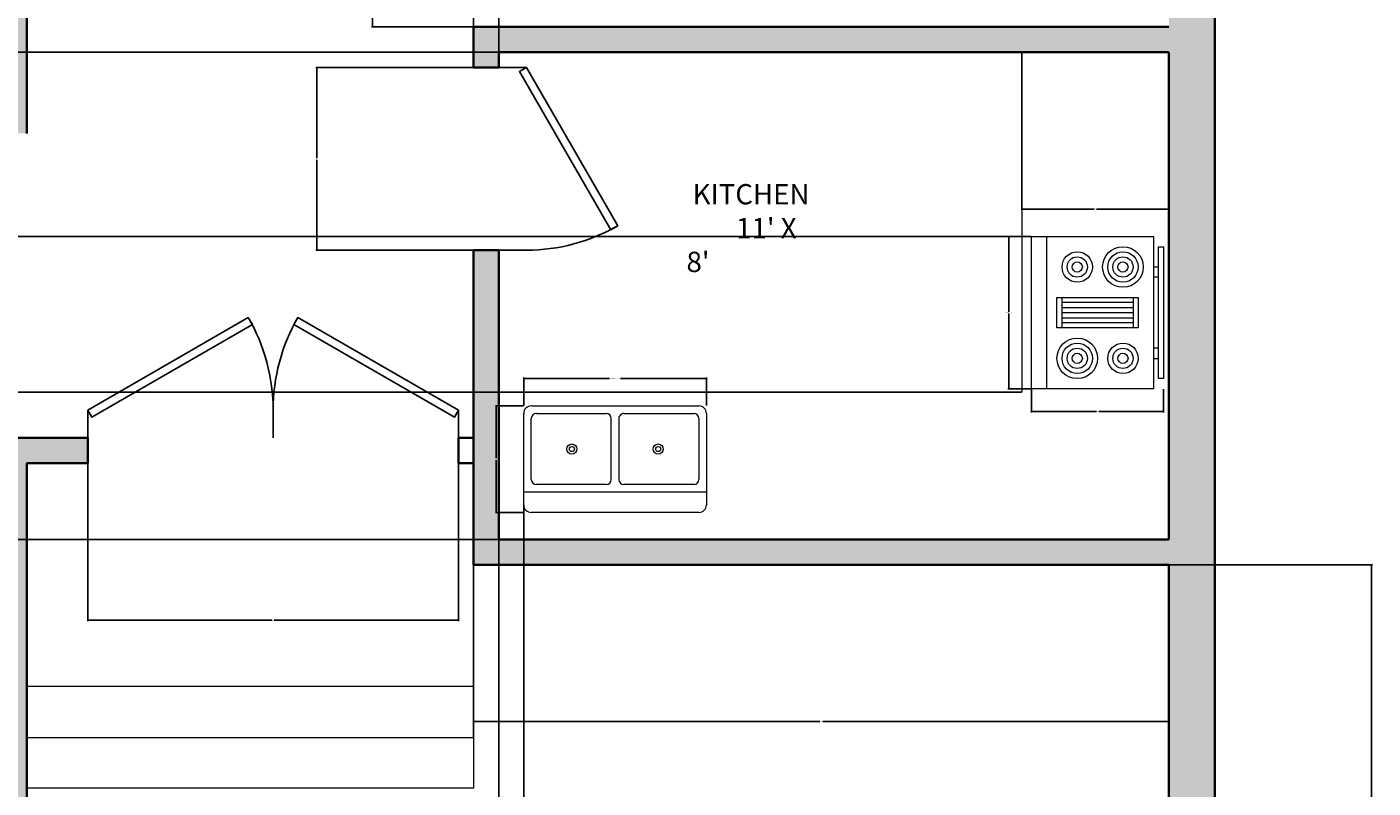
# Model space of a CAD drawing. Units: inches. Extents: x -30 to 437, y -29 to 647.
# Tile 6 of 15: x 172 to 437, y 105 to 255. Entities that reach past the tile are written whole.
import ezdxf

# ---------------------------------------------------------------- set-up
doc = ezdxf.new("R2010")
doc.units = ezdxf.units.IN
doc.header["$MEASUREMENT"] = 0
for name, color, linetype, lineweight in [('A-ANNO-DIMS', 2, 'Continuous', 18), ('A-AREA-IDEN', 7, 'Continuous', 18), ('A-FLOR-STRS', 7, 'Continuous', 18), ('A-WALL', 7, 'Continuous', 35), ('doors', 40, 'Continuous', 25), ('kitchen', 181, 'Continuous', 18)]:
    doc.layers.add(name, color=color, linetype=linetype, lineweight=lineweight)
doc.layers.add('A-WALL-PATT', color=251, linetype='Continuous', lineweight=13, true_color=0x636466)
doc.styles.get("Standard").update_dxf_attribs({"font": 'arial.ttf'})
doc.dimstyles.get("Standard").update_dxf_attribs({"dimtxt": 0.18, "dimasz": 0.18, "dimexe": 0.18, "dimexo": 0.0625, "dimgap": 0.09, "dimtad": 0, "dimtih": 1, "dimtoh": 1, "dimdec": 4, "dimzin": 0, "dimdsep": 46, "dimtxsty": 'Standard', "dimcen": 0.09, "dimadec": 0, "dimazin": 0, "dimtfac": 1, "dimtdec": 4, "dimtofl": 0, "dimtmove": 0, "dimatfit": 3, "dimfxl": 1, "dimtolj": 1, "dimtzin": 0, "dimarcsym": 0})

# ---------------------------------------------------------------- blocks, each defined once
blk = doc.blocks.new('*U6')
for p, q in [((0, 0), (0, -6)), ((40, 0), (40, -6))]:
    blk.add_line(p, q)
blk.add_lwpolyline([(0, 0), (34.64, 20), (35.52, 18.48), (0.87, -1.52)], close=True)
blk.add_arc((0, 0), 40, 0, 30)
blk = doc.blocks.new('Range-Oven - 30 in top')
for p, q in [((0, -3), (30, -3)), ((12, -6), (18, -6)), ((13, -20), (13, -6)), ((14, -6), (14, -20)), ((15, -20), (15, -6)), ((16, -6), (16, -20)), ((17, -20), (17, -6)), ((18, -20), (12, -20)), ((6, -24), (6, -25)), ((8, -25), (8, -24)), ((22, -25), (22, -24)), ((24, -24), (24, -25))]:
    blk.add_line(p, q)
for points in [[(0, -24), (0, 0), (30, 0), (30, -24)], [(12, -21), (12, -5), (18, -5), (18, -21)], [(2, -26), (2, -25), (28, -25), (28, -26)]]:
    blk.add_lwpolyline(points, close=True)
for centre, radius in [((6, -9), 4), ((6, -9), 3), ((6, -9), 2), ((24, -9), 3), ((24, -9), 2), ((6, -9), 1), ((24, -9), 1), ((6, -18), 3), ((24, -18), 4), ((24, -18), 3), ((6, -18), 2), ((6, -18), 1), ((24, -18), 2), ((24, -18), 1)]:
    blk.add_circle(centre, radius)
blk = doc.blocks.new('Sink-double - 36 in top')
for p, q in [((-18, -4), (18, -4)), ((-0.75, -18.5), (-0.75, -6.5)), ((0.75, -6.5), (0.75, -18.5))]:
    blk.add_line(p, q)
for points in [[(-16.5, 0), (16.5, 0)], [(-18, -19.5), (-18, -1.5)], [(18, -1.5), (18, -19.5)], [(-16.5, -18.5), (-16.5, -6.5)], [(-15.5, -5.5), (-1.75, -5.5)], [(1.75, -5.5), (15.5, -5.5)], [(16.5, -6.5), (16.5, -18.5)], [(16.5, -21), (-16.5, -21)], [(-1.75, -19.5), (-15.5, -19.5)], [(15.5, -19.5), (1.75, -19.5)]]:
    blk.add_lwpolyline(points)
for centre, radius in [((-8.5, -12.5), 1), ((-8.5, -12.5), 0.5), ((8.5, -12.5), 1), ((8.5, -12.5), 0.5)]:
    blk.add_circle(centre, radius)
for centre, radius, start, end in [((-16.5, -1.5), 1.5, 90, 180), ((16.5, -1.5), 1.5, 0, 90), ((-15.5, -6.5), 1, 90, 180), ((-1.75, -6.5), 1, 0, 90), ((1.75, -6.5), 1, 90, 180), ((15.5, -6.5), 1, 0, 90), ((-15.5, -18.5), 1, 180, 270), ((-1.75, -18.5), 1, 270, 0), ((1.75, -18.5), 1, 180, 270), ((15.5, -18.5), 1, 270, 0), ((-16.5, -19.5), 1.5, 180, 270), ((16.5, -19.5), 1.5, 270, 0)]:
    blk.add_arc(centre, radius, start, end)
blk = doc.blocks.new('*D21')
at = {"layer": 'A-ANNO-DIMS', "color": 0, "lineweight": -2, "transparency": 16777216}
for p, q in [((369.54, 213.24), (364.93, 213.24)), ((365.11, 213.06), (365.11, 198.42)), ((365.11, 183.42), (365.11, 198.05)), ((369.54, 183.24), (364.93, 183.24))]:
    blk.add_line(p, q, dxfattribs=at)
at = {"layer": 'A-ANNO-DIMS', "color": 0, "transparency": 16777216}
for points in [[(365.08, 213.06), (365.14, 213.06), (365.11, 213.24)], [(365.08, 183.42), (365.14, 183.42), (365.11, 183.24)]]:
    blk.add_solid(points, dxfattribs=at)
at = {"layer": 'Defpoints', "color": 0, "transparency": 16777216}
for p in [(365.11, 213.24), (369.61, 213.24), (369.61, 183.24)]:
    blk.add_point(p, dxfattribs=at)
at = {"layer": 'A-ANNO-DIMS', "color": 0, "transparency": 16777216, "insert": (365.11, 198.24), "char_height": 0.18, "attachment_point": 5}
blk.add_mtext('\\A1;RANGE 30', dxfattribs=at)
blk = doc.blocks.new('*D22')
at = {"layer": 'A-ANNO-DIMS', "color": 0, "lineweight": -2, "transparency": 16777216}
for p, q in [((369.61, 183.17), (369.61, 178.56)), ((395.61, 183.17), (395.61, 178.56)), ((369.79, 178.74), (382.39, 178.74)), ((395.43, 178.74), (382.83, 178.74))]:
    blk.add_line(p, q, dxfattribs=at)
at = {"layer": 'A-ANNO-DIMS', "color": 0, "transparency": 16777216}
for points in [[(369.79, 178.77), (369.79, 178.71), (369.61, 178.74)], [(395.43, 178.77), (395.43, 178.71), (395.61, 178.74)]]:
    blk.add_solid(points, dxfattribs=at)
at = {"layer": 'Defpoints', "color": 0, "transparency": 16777216}
for p in [(369.61, 183.24), (395.61, 183.24), (369.61, 178.74)]:
    blk.add_point(p, dxfattribs=at)
at = {"layer": 'A-ANNO-DIMS', "color": 0, "transparency": 16777216, "insert": (382.61, 178.74), "char_height": 0.18, "attachment_point": 5}
blk.add_mtext('\\A1;26', dxfattribs=at)
blk = doc.blocks.new('*D23')
at = {"layer": 'A-ANNO-DIMS', "color": 0, "lineweight": -2, "transparency": 16777216}
for p, q in [((269.54, 179.93), (269.54, 185.45)), ((269.72, 185.27), (286.45, 185.27)), ((305.36, 185.27), (288.64, 185.27)), ((305.54, 179.93), (305.54, 185.45))]:
    blk.add_line(p, q, dxfattribs=at)
at = {"layer": 'A-ANNO-DIMS', "color": 0, "transparency": 16777216}
for points in [[(269.72, 185.3), (269.72, 185.24), (269.54, 185.27)], [(305.36, 185.3), (305.36, 185.24), (305.54, 185.27)]]:
    blk.add_solid(points, dxfattribs=at)
at = {"layer": 'Defpoints', "color": 0, "transparency": 16777216}
for p in [(269.54, 185.27), (269.54, 179.87), (305.54, 179.87)]:
    blk.add_point(p, dxfattribs=at)
at = {"layer": 'A-ANNO-DIMS', "color": 0, "transparency": 16777216, "insert": (287.54, 185.27), "char_height": 0.18, "attachment_point": 5}
blk.add_mtext('\\A1;DOUBLE SINK 36', dxfattribs=at)
blk = doc.blocks.new('*D24')
at = {"layer": 'A-ANNO-DIMS', "color": 0, "lineweight": -2, "transparency": 16777216}
for p, q in [((269.48, 179.87), (263.96, 179.87)), ((264.14, 179.69), (264.14, 169.55)), ((264.14, 159.05), (264.14, 169.19)), ((269.48, 158.87), (263.96, 158.87))]:
    blk.add_line(p, q, dxfattribs=at)
at = {"layer": 'A-ANNO-DIMS', "color": 0, "transparency": 16777216}
for points in [[(264.11, 179.69), (264.17, 179.69), (264.14, 179.87)], [(264.11, 159.05), (264.17, 159.05), (264.14, 158.87)]]:
    blk.add_solid(points, dxfattribs=at)
at = {"layer": 'Defpoints', "color": 0, "transparency": 16777216}
for p in [(269.54, 179.87), (264.14, 158.87), (269.54, 158.87)]:
    blk.add_point(p, dxfattribs=at)
at = {"layer": 'A-ANNO-DIMS', "color": 0, "transparency": 16777216, "insert": (264.14, 169.37), "char_height": 0.18, "attachment_point": 5}
blk.add_mtext('\\A1;21', dxfattribs=at)
blk = doc.blocks.new('*D37')
at = {"layer": 'A-ANNO-DIMS', "color": 0, "lineweight": -2, "transparency": 16777216}
for p, q in [((259.67, 148.48), (259.67, 117.47)), ((396.67, 148.48), (396.67, 117.47)), ((259.85, 117.65), (327.89, 117.65)), ((396.49, 117.65), (328.45, 117.65))]:
    blk.add_line(p, q, dxfattribs=at)
at = {"layer": 'A-ANNO-DIMS', "color": 0, "transparency": 16777216}
for points in [[(259.85, 117.68), (259.85, 117.62), (259.67, 117.65)], [(396.49, 117.68), (396.49, 117.62), (396.67, 117.65)]]:
    blk.add_solid(points, dxfattribs=at)
at = {"layer": 'Defpoints', "color": 0, "transparency": 16777216}
for p in [(259.67, 148.55), (396.67, 148.55), (259.67, 117.65)]:
    blk.add_point(p, dxfattribs=at)
at = {"layer": 'A-ANNO-DIMS', "color": 0, "transparency": 16777216, "insert": (328.17, 117.65), "char_height": 0.18, "attachment_point": 5}
blk.add_mtext('\\A1;137', dxfattribs=at)
blk = doc.blocks.new('*D39')
at = {"layer": 'A-ANNO-DIMS', "color": 0, "lineweight": -2, "transparency": 16777216}
for p, q in [((396.74, 148.55), (436.75, 148.55)), ((436.57, 148.37), (436.57, 75.48)), ((436.57, 2.23), (436.57, 75.12)), ((396.74, 2.05), (436.75, 2.05))]:
    blk.add_line(p, q, dxfattribs=at)
at = {"layer": 'A-ANNO-DIMS', "color": 0, "transparency": 16777216}
for points in [[(436.54, 148.37), (436.6, 148.37), (436.57, 148.55)], [(436.54, 2.23), (436.6, 2.23), (436.57, 2.05)]]:
    blk.add_solid(points, dxfattribs=at)
at = {"layer": 'Defpoints', "color": 0, "transparency": 16777216}
for p in [(396.67, 148.55), (436.57, 148.55), (396.67, 2.05)]:
    blk.add_point(p, dxfattribs=at)
at = {"layer": 'A-ANNO-DIMS', "color": 0, "transparency": 16777216, "insert": (436.57, 75.3), "char_height": 0.18, "attachment_point": 5}
blk.add_mtext('\\A1;146.5', dxfattribs=at)
blk = doc.blocks.new('*D41')
at = {"layer": 'A-ANNO-DIMS', "color": 0, "lineweight": -2, "transparency": 16777216}
for p, q in [((183.67, 168.48), (183.67, 137.47)), ((256.67, 168.48), (256.67, 137.47)), ((183.85, 137.65), (219.96, 137.65)), ((256.49, 137.65), (220.39, 137.65))]:
    blk.add_line(p, q, dxfattribs=at)
at = {"layer": 'A-ANNO-DIMS', "color": 0, "transparency": 16777216}
for points in [[(183.85, 137.68), (183.85, 137.62), (183.67, 137.65)], [(256.49, 137.68), (256.49, 137.62), (256.67, 137.65)]]:
    blk.add_solid(points, dxfattribs=at)
at = {"layer": 'Defpoints', "color": 0, "transparency": 16777216}
for p in [(183.67, 168.55), (256.67, 168.55), (183.67, 137.65)]:
    blk.add_point(p, dxfattribs=at)
at = {"layer": 'A-ANNO-DIMS', "color": 0, "transparency": 16777216, "insert": (220.17, 137.65), "char_height": 0.18, "attachment_point": 5}
blk.add_mtext('\\A1;73', dxfattribs=at)
blk = doc.blocks.new('*D45')
at = {"layer": 'A-ANNO-DIMS', "color": 0, "lineweight": -2, "transparency": 16777216}
for p, q in [((270.61, 290.55), (239.59, 290.55)), ((239.77, 290.37), (239.77, 272.73)), ((239.77, 254.73), (239.77, 272.37)), ((270.61, 254.55), (239.59, 254.55))]:
    blk.add_line(p, q, dxfattribs=at)
at = {"layer": 'A-ANNO-DIMS', "color": 0, "transparency": 16777216}
for points in [[(239.74, 290.37), (239.8, 290.37), (239.77, 290.55)], [(239.74, 254.73), (239.8, 254.73), (239.77, 254.55)]]:
    blk.add_solid(points, dxfattribs=at)
at = {"layer": 'Defpoints', "color": 0, "transparency": 16777216}
for p in [(239.77, 290.55), (270.67, 290.55), (270.67, 254.55)]:
    blk.add_point(p, dxfattribs=at)
at = {"layer": 'A-ANNO-DIMS', "color": 0, "transparency": 16777216, "insert": (239.77, 272.55), "char_height": 0.18, "attachment_point": 5}
blk.add_mtext('\\A1;36', dxfattribs=at)
blk = doc.blocks.new('*D51')
at = {"layer": 'A-ANNO-DIMS', "color": 0, "lineweight": -2, "transparency": 16777216}
for p, q in [((367.67, 249.48), (367.67, 218.47)), ((396.67, 249.48), (396.67, 218.47)), ((367.85, 218.65), (381.95, 218.65)), ((396.49, 218.65), (382.39, 218.65))]:
    blk.add_line(p, q, dxfattribs=at)
at = {"layer": 'A-ANNO-DIMS', "color": 0, "transparency": 16777216}
for points in [[(367.85, 218.68), (367.85, 218.62), (367.67, 218.65)], [(396.49, 218.68), (396.49, 218.62), (396.67, 218.65)]]:
    blk.add_solid(points, dxfattribs=at)
at = {"layer": 'Defpoints', "color": 0, "transparency": 16777216}
for p in [(367.67, 249.55), (396.67, 249.55), (367.67, 218.65)]:
    blk.add_point(p, dxfattribs=at)
at = {"layer": 'A-ANNO-DIMS', "color": 0, "transparency": 16777216, "insert": (382.17, 218.65), "char_height": 0.18, "attachment_point": 5}
blk.add_mtext('\\A1;29', dxfattribs=at)
blk = doc.blocks.new('*D52')
at = {"layer": 'A-ANNO-DIMS', "color": 0, "lineweight": -2, "transparency": 16777216}
for p, q in [((367.61, 182.55), (-29.41, 182.55)), ((-29.23, 182.37), (-29.23, 168.23)), ((-29.23, 153.73), (-29.23, 167.87)), ((396.61, 153.55), (-29.41, 153.55))]:
    blk.add_line(p, q, dxfattribs=at)
at = {"layer": 'A-ANNO-DIMS', "color": 0, "transparency": 16777216}
for points in [[(-29.26, 182.37), (-29.2, 182.37), (-29.23, 182.55)], [(-29.26, 153.73), (-29.2, 153.73), (-29.23, 153.55)]]:
    blk.add_solid(points, dxfattribs=at)
at = {"layer": 'Defpoints', "color": 0, "transparency": 16777216}
for p in [(367.67, 182.55), (-29.23, 153.55), (396.67, 153.55)]:
    blk.add_point(p, dxfattribs=at)
at = {"layer": 'A-ANNO-DIMS', "color": 0, "transparency": 16777216, "insert": (-29.23, 168.05), "char_height": 0.18, "attachment_point": 5}
blk.add_mtext('\\A1;29', dxfattribs=at)
blk = doc.blocks.new('*D53')
at = {"layer": 'A-ANNO-DIMS', "color": 0, "lineweight": -2, "transparency": 16777216}
for p, q in [((259.61, 246.55), (228.59, 246.55)), ((228.77, 246.37), (228.77, 228.73)), ((228.77, 210.73), (228.77, 228.37)), ((259.61, 210.55), (228.59, 210.55))]:
    blk.add_line(p, q, dxfattribs=at)
at = {"layer": 'A-ANNO-DIMS', "color": 0, "transparency": 16777216}
for points in [[(228.74, 246.37), (228.8, 246.37), (228.77, 246.55)], [(228.74, 210.73), (228.8, 210.73), (228.77, 210.55)]]:
    blk.add_solid(points, dxfattribs=at)
at = {"layer": 'Defpoints', "color": 0, "transparency": 16777216}
for p in [(228.77, 246.55), (259.67, 246.55), (259.67, 210.55)]:
    blk.add_point(p, dxfattribs=at)
at = {"layer": 'A-ANNO-DIMS', "color": 0, "transparency": 16777216, "insert": (228.77, 228.55), "char_height": 0.18, "attachment_point": 5}
blk.add_mtext('\\A1;36', dxfattribs=at)
blk = doc.blocks.new('*D54')
at = {"layer": 'A-ANNO-DIMS', "color": 0, "lineweight": -2, "transparency": 16777216}
for p, q in [((259.67, 254.61), (259.67, 646.63)), ((259.85, 646.45), (262.02, 646.45)), ((264.49, 646.45), (262.32, 646.45)), ((264.67, 249.61), (264.67, 646.63))]:
    blk.add_line(p, q, dxfattribs=at)
at = {"layer": 'A-ANNO-DIMS', "color": 0, "transparency": 16777216}
for points in [[(259.85, 646.48), (259.85, 646.42), (259.67, 646.45)], [(264.49, 646.48), (264.49, 646.42), (264.67, 646.45)]]:
    blk.add_solid(points, dxfattribs=at)
at = {"layer": 'Defpoints', "color": 0, "transparency": 16777216}
for p in [(259.67, 646.45), (259.67, 254.55), (264.67, 249.55)]:
    blk.add_point(p, dxfattribs=at)
at = {"layer": 'A-ANNO-DIMS', "color": 0, "transparency": 16777216, "insert": (262.17, 646.45), "char_height": 0.18, "attachment_point": 5}
blk.add_mtext('\\A1;5', dxfattribs=at)
blk = doc.blocks.new('*D55')
at = {"layer": 'A-ANNO-DIMS', "color": 0, "lineweight": -2, "transparency": 16777216}
for p, q in [((367.61, 249.55), (-29.41, 249.55)), ((-29.23, 249.37), (-29.23, 231.57)), ((-29.23, 213.42), (-29.23, 231.21)), ((369.54, 213.24), (-29.41, 213.24))]:
    blk.add_line(p, q, dxfattribs=at)
at = {"layer": 'A-ANNO-DIMS', "color": 0, "transparency": 16777216}
for points in [[(-29.26, 249.37), (-29.2, 249.37), (-29.23, 249.55)], [(-29.26, 213.42), (-29.2, 213.42), (-29.23, 213.24)]]:
    blk.add_solid(points, dxfattribs=at)
at = {"layer": 'Defpoints', "color": 0, "transparency": 16777216}
for p in [(-29.23, 249.55), (367.67, 249.55), (369.61, 213.24)]:
    blk.add_point(p, dxfattribs=at)
at = {"layer": 'A-ANNO-DIMS', "color": 0, "transparency": 16777216, "insert": (-29.23, 231.39), "char_height": 0.18, "attachment_point": 5}
blk.add_mtext('\\A1;36.31', dxfattribs=at)
blk = doc.blocks.new('*D56')
at = {"layer": 'A-ANNO-DIMS', "color": 0, "lineweight": -2, "transparency": 16777216}
for p, q in [((269.54, 160.3), (269.54, -29.03)), ((264.67, 153.48), (264.67, -29.03)), ((264.85, -28.85), (266.78, -28.85)), ((269.36, -28.85), (267.44, -28.85))]:
    blk.add_line(p, q, dxfattribs=at)
at = {"layer": 'A-ANNO-DIMS', "color": 0, "transparency": 16777216}
for points in [[(264.85, -28.82), (264.85, -28.88), (264.67, -28.85)], [(269.36, -28.82), (269.36, -28.88), (269.54, -28.85)]]:
    blk.add_solid(points, dxfattribs=at)
at = {"layer": 'Defpoints', "color": 0, "transparency": 16777216}
for p in [(269.54, 160.37), (264.67, 153.55), (269.54, -28.85)]:
    blk.add_point(p, dxfattribs=at)
at = {"layer": 'A-ANNO-DIMS', "color": 0, "transparency": 16777216, "insert": (267.11, -28.85), "char_height": 0.18, "attachment_point": 5}
blk.add_mtext('\\A1;4.87', dxfattribs=at)

msp = doc.modelspace()

# ---------------------------------------------------------------- hatches: boundary and pattern name
at = {"layer": 'A-WALL-PATT'}
h = msp.add_hatch(color=256, dxfattribs=at)
h.dxf.hatch_style = 1
h.paths.add_polyline_path([(393.6054, 183.2352), (369.6054, 183.2352), (369.6054, 213.2352), (393.6054, 213.2352), (393.6054, 207.2352), (394.6054, 207.2352), (394.6054, 211.2352), (395.6054, 211.2352), (395.6054, 185.2352), (394.6054, 185.2352), (394.6054, 189.2352), (393.6054, 189.2352)], flags=0)
h.paths.add_polyline_path([(384.6054, 189.2352, -1), (390.6054, 189.2352, -1)], flags=0)
h.paths.add_polyline_path([(385.6054, 189.2352, -1), (389.6054, 189.2352, -1)], flags=0)
h.paths.add_polyline_path([(374.6054, 189.2352, -1), (382.6054, 189.2352, -1)], flags=0)
h.paths.add_polyline_path([(386.6054, 189.2352, -1), (388.6054, 189.2352, -1)], flags=0)
h.paths.add_polyline_path([(375.6054, 189.2352, -1), (381.6054, 189.2352, -1)], flags=0)
h.paths.add_polyline_path([(376.6054, 189.2352, -1), (380.6054, 189.2352, -1)], flags=0)
h.paths.add_polyline_path([(377.6054, 189.2352, -1), (379.6054, 189.2352, -1)], flags=0)
h.paths.add_polyline_path([(390.6054, 195.2352), (374.6054, 195.2352), (374.6054, 201.2352), (390.6054, 201.2352)], flags=0)
h.paths.add_polyline_path([(389.6054, 196.2352), (375.6054, 196.2352), (375.6054, 200.2352), (389.6054, 200.2352)], flags=0)
h.paths.add_polyline_path([(383.6054, 207.2352, -1), (391.6054, 207.2352, -1)], flags=0)
h.paths.add_polyline_path([(384.6054, 207.2352, -1), (390.6054, 207.2352, -1)], flags=0)
h.paths.add_polyline_path([(385.6054, 207.2352, -1), (389.6054, 207.2352, -1)], flags=0)
h.paths.add_polyline_path([(386.6054, 207.2352, -1), (388.6054, 207.2352, -1)], flags=0)
h.paths.add_polyline_path([(375.6054, 207.2352, -1), (381.6054, 207.2352, -1)], flags=0)
h.paths.add_polyline_path([(376.6054, 207.2352, -1), (380.6054, 207.2352, -1)], flags=0)
h.paths.add_polyline_path([(377.6054, 207.2352, -1), (379.6054, 207.2352, -1)], flags=0)
h.paths.add_polyline_path([(305.5437, 160.3663, -0.41421356), (304.0437, 158.8663), (271.0437, 158.8663, -0.41421356), (269.5437, 160.3663), (269.5437, 178.3663, -0.41421356), (271.0437, 179.8663), (304.0437, 179.8663, -0.41421356), (305.5437, 178.3663)], flags=0)
h.paths.add_polyline_path([(304.0437, 165.3663, -0.41421356), (303.0437, 164.3663), (289.2937, 164.3663, -0.41421356), (288.2937, 165.3663), (288.2937, 177.3663, -0.41421356), (289.2937, 178.3663), (303.0437, 178.3663, -0.41421356), (304.0437, 177.3663)], flags=0)
h.paths.add_polyline_path([(296.5437, 171.3663, -1), (295.5437, 171.3663, -1)], flags=0)
h.paths.add_polyline_path([(286.7937, 165.3663, -0.41421356), (285.7937, 164.3663), (272.0437, 164.3663, -0.41421356), (271.0437, 165.3663), (271.0437, 177.3663, -0.41421356), (272.0437, 178.3663), (285.7937, 178.3663, -0.41421356), (286.7937, 177.3663)], flags=0)
h.paths.add_polyline_path([(279.5437, 171.3663, -1), (278.5437, 171.3663, -1)], flags=0)
h.paths.add_polyline_path([(360.6737, 290.5474), (360.6737, 300.5474), (396.6737, 300.5474), (396.6737, 290.5474)], flags=0)
h.paths.add_polyline_path([(259.6737, 124.5474), (259.6737, 114.5474), (171.6737, 114.5474), (171.6737, 124.5474)], flags=0)
h.paths.add_polyline_path([(288.0737, 215.3705), (286.7097, 214.583), (268.7097, 245.7599), (270.0737, 246.5474)], flags=0)
h.paths.add_polyline_path([(259.6737, 168.5474), (256.6737, 168.5474), (256.6737, 173.5474), (256.6737, 179.0224), (255.8753, 177.6395), (224.2956, 195.872, 0.12053744), (220.1737, 179.0224, 0.12053744), (216.0518, 195.872), (184.4721, 177.6395), (183.6737, 179.0224), (215.2836, 197.2724), (216.0821, 195.8895), (216.0518, 195.872, -0.12053744), (220.1737, 179.0224, -0.12053744), (224.2956, 195.872), (224.2653, 195.8895), (225.0638, 197.2724), (256.6737, 179.0224), (256.6737, 173.5474), (259.6737, 173.5474)], flags=0)
h.paths.add_polyline_path([(386.7943, 325.4601), (372.6871, 325.4601), (372.6871, 339.5673), (386.7943, 339.5673)], flags=0)
h.paths.add_polyline_path([(359.5875, 343.7429), (357.7905, 343.7429), (357.7905, 327.9179), (359.3933, 327.9179, 0.41420885), (361.5302, 330.0549), (361.5302, 341.8434, 0.41436161)], flags=0)
h.paths.add_polyline_path([(341.7887, 323.1235, -0.11921667), (340.7839, 323.1235)], flags=0)
h.paths.add_polyline_path([(379.6332, 328.8632), (379.6332, 332.2699), (376.0992, 332.2699, 0.39427733)], flags=0)
h.paths.add_polyline_path([(375.5299, 332.459, -1), (383.8511, 332.459, -1)], flags=0)
h.paths.add_polyline_path([(388.9363, 344.7425), (372.5309, 344.7425, -0.41421356), (370.394, 346.8794), (370.394, 347.5594, -0.39085173), (372.3472, 349.7005, -0.43951011), (370.394, 351.4933), (370.394, 365.1894, -0.40305452), (372.2191, 367.1298, -0.41839453), (370.394, 368.9291), (370.394, 382.6251, -0.40885826), (372.2519, 384.5722, -0.42377324), (370.394, 386.3707), (370.394, 400.0667, -0.38660687), (372.1327, 402.0094), (372.531, 402.0094, -0.41421834), (370.394, 404.1464), (370.394, 404.7778, -0.41420891), (372.5309, 406.9147), (388.9363, 406.9147, -0.41421821), (391.0733, 404.7778), (391.0733, 346.8794, -0.41421356)], flags=0)
edge = h.paths.add_edge_path(flags=0)
edge.add_spline(control_points=[(349.3585, 363.204), (349.0859, 363.204), (348.8133, 363.2227), (348.2712, 363.2973), (348.0016, 363.3531), (347.3533, 363.5328), (346.9776, 363.6755), (346.2445, 364.0308), (345.887, 364.2432), (345.1953, 364.7329), (344.8611, 365.0101), (344.2197, 365.6237), (343.9125, 365.9603), (343.211, 366.8336), (342.8313, 367.3965), (342.1401, 368.6117), (341.8286, 369.2641), (341.2807, 370.64), (341.0443, 371.3636), (340.6522, 372.8619), (340.4964, 373.6367), (340.2695, 375.2158), (340.1983, 376.0203), (340.142, 377.6365), (340.157, 378.4483), (340.2729, 380.0567), (340.3738, 380.8533), (340.6589, 382.4093), (340.8432, 383.1686), (341.2906, 384.629), (341.5538, 385.3301), (342.1531, 386.6544), (342.4891, 387.2776), (343.2266, 388.4288), (343.6281, 388.9567), (344.4879, 389.9012), (344.9463, 390.3178), (345.7981, 390.9428), (346.182, 391.1771), (346.9712, 391.5648), (347.3766, 391.7182), (348.2004, 391.9387), (348.6189, 392.0058), (349.4588, 392.0508), (349.8801, 392.0288), (350.7146, 391.8966), (351.1278, 391.7865), (351.9366, 391.4822), (352.3323, 391.2882), (353.0989, 390.8223), (353.4699, 390.5504), (354.1819, 389.9355), (354.5229, 389.5924), (355.1706, 388.8418), (355.4772, 388.4343), (356.1315, 387.4422), (356.4671, 386.8397), (357.0692, 385.5581), (357.3356, 384.879), (357.7933, 383.4624), (357.9846, 382.725), (358.2875, 381.2112), (358.3992, 380.4349), (358.5404, 378.8643), (358.5699, 378.0699), (358.546, 376.4841), (358.4926, 375.6928), (358.3042, 374.1343), (358.1692, 373.3672), (357.8207, 371.8774), (357.6072, 371.1549), (357.1067, 369.7735), (356.8196, 369.1148), (356.1782, 367.8787), (355.8238, 367.3013), (355.0551, 366.244), (354.6408, 365.7641), (353.7607, 364.9161), (353.2948, 364.5481), (352.445, 364.0149), (352.0701, 363.822), (351.3034, 363.5117), (350.9116, 363.3943), (350.1325, 363.2418), (349.7455, 363.204), (349.3585, 363.204)], knot_values=[3.14159265, 3.14159265, 3.14159265, 3.14159265, 3.22691715, 3.22691715, 3.31224165, 3.31224165, 3.43426671, 3.43426671, 3.55629177, 3.55629177, 3.67831683, 3.67831683, 3.8003419, 3.8003419, 3.97157384, 3.97157384, 4.14280577, 4.14280577, 4.31403771, 4.31403771, 4.48526965, 4.48526965, 4.65650159, 4.65650159, 4.82773353, 4.82773353, 4.99896547, 4.99896547, 5.1701974, 5.1701974, 5.34142934, 5.34142934, 5.51266128, 5.51266128, 5.68389322, 5.68389322, 5.85512516, 5.85512516, 5.98669107, 5.98669107, 6.11825699, 6.11825699, 6.24982291, 6.24982291, 6.38138882, 6.38138882, 6.51295474, 6.51295474, 6.64452065, 6.64452065, 6.77608657, 6.77608657, 6.90765249, 6.90765249, 7.0392184, 7.0392184, 7.20701563, 7.20701563, 7.37481286, 7.37481286, 7.54261009, 7.54261009, 7.71040732, 7.71040732, 7.87820455, 7.87820455, 8.04600178, 8.04600178, 8.21379901, 8.21379901, 8.38159624, 8.38159624, 8.54939347, 8.54939347, 8.7171907, 8.7171907, 8.88498794, 8.88498794, 9.05278517, 9.05278517, 9.17820699, 9.17820699, 9.30362881, 9.30362881, 9.42477796, 9.42477796, 9.42477796, 9.42477796], degree=3, periodic=0)
edge.add_line((341.1696, 384.3006), (341.2012, 384.2808))
edge = h.paths.add_edge_path(flags=0)
edge.add_line((344.3353, 388.7801), (344.317, 388.7915))
edge.add_ellipse((349.3585, 377.6204), major_axis=(0, -13.7895), ratio=0.62186025, start_angle=-244.867444, end_angle=-124.769923)
h.paths.add_polyline_path([(163.6737, 163.1474), (132.4968, 145.1474), (131.7093, 146.5114), (162.8862, 164.5114)], flags=0)
h.paths.add_polyline_path([(366.4355, 409.0896, -0.41423669), (364.2985, 406.9525, -0.4913499), (361.5302, 408.8973), (361.5302, 420.6405, 0.41421356), (359.3932, 422.7775), (357.7905, 422.7775), (357.7905, 406.9525), (359.6317, 406.9525, 0.42741026), (361.5332, 408.9757, 0.39869469), (363.6672, 406.9525, 0.51958103), (366.4355, 409.0895)], flags=0)
h.paths.add_polyline_path([(386.7943, 410.9671), (372.6871, 410.9671), (372.6871, 425.0742), (386.7943, 425.0742)], flags=0)
h.paths.add_polyline_path([(379.6332, 414.3701), (379.6332, 417.7768), (376.0992, 417.7768, 0.39427733)], flags=0)
h.paths.add_polyline_path([(375.5299, 417.966, -1), (383.8511, 417.966, -1)], flags=0)
h.paths.add_polyline_path([(150.0377, 351.583), (148.6737, 352.3705), (166.6737, 383.5474), (168.0377, 382.7599)], flags=0)
h.paths.add_polyline_path([(91.6737, 234.1974), (66.559, 219.6974), (65.9246, 220.7962), (91.0393, 235.2962)], flags=0)
h.paths.add_polyline_path([(255.4612, 443.5834), (254.6737, 444.9474), (285.8506, 462.9474), (286.6381, 461.5834)], flags=0)
h.paths.add_polyline_path([(176.2737, 394.5474), (158.2737, 425.7243), (159.6377, 426.5118), (177.6377, 395.3349)], flags=0)
h.paths.add_polyline_path([(243.6737, 439.5474), (243.0393, 438.4486), (217.9246, 452.9486), (218.559, 454.0474)], flags=0)
h.paths.add_polyline_path([(38.1264, 269.8429), (40.2408, 269.8429), (40.2408, 270.3508), (38.1264, 270.3508)], flags=0)
h.paths.add_polyline_path([(75.7157, 289.9439), (40.2408, 289.9439), (38.1264, 289.6524), (40.2408, 289.6524)], flags=0)
h.paths.add_polyline_path([(75.7157, 270.0846), (77.6447, 270.0846), (77.6697, 270.1626), (75.7175, 270.1626)], flags=0)
h.paths.add_polyline_path([(80.5373, 293.3002), (33.0467, 293.3002), (13.5054, 293.3002), (13.5054, 351.9244), (29.7898, 351.9244), (80.5373, 351.9244)], flags=0)
h.paths.add_polyline_path([(46.0261, 212.466, -0.50131678), (27.1651, 207.5106), (21.165, 209.5107), (21.165, 206.5107), (22.665, 206.5107), (22.665, 203.5107), (21.165, 203.5107), (21.165, 203.0107), (13.165, 203.0107), (13.165, 224.0107), (21.165, 224.0107), (21.165, 217.5107), (27.1649, 219.5106, -0.50132349), (46.0261, 214.5554, -0.13289091)], flags=0)
h.paths.add_polyline_path([(44.688, 211.8666, -0.48007965), (27.165, 209.5107), (27.165, 217.5107, -0.4800795), (44.688, 215.1547, -0.21500378)], flags=0)
h.paths.add_polyline_path([(19.415, 204.0107), (15.165, 204.0107, -0.41421356), (14.165, 204.7607), (14.165, 222.0107, -0.41421356), (14.915, 223.0107), (19.165, 223.0107, -0.41421356), (20.165, 222.2607), (20.165, 205.0107, -0.41421356)], flags=0)
h.paths.add_polyline_path([(32.7608, 269.0719), (31.8439, 269.0719), (31.8439, 268.6134), (13.5054, 268.6134), (13.5054, 291.5366), (31.8439, 291.5366), (32.7608, 291.0781), (32.7608, 280.9919, -1), (32.7608, 279.1581)], flags=0)
h.paths.add_polyline_path([(40.2408, 360.1436), (38.1264, 360.1436), (38.1264, 359.6357), (40.2408, 359.6357)], flags=0)
h.paths.add_polyline_path([(75.7157, 355.2807), (40.2408, 355.2807), (38.1264, 355.5722), (40.2408, 355.5722), (40.2408, 355.2807), (75.7157, 355.2807), (75.7157, 375.5982), (40.2408, 375.5982), (38.1264, 375.3817), (40.2408, 375.3817), (40.2408, 375.5982), (75.7157, 375.5982), (77.9733, 375.062), (75.7175, 375.062), (75.7175, 374.554)], flags=0)
h.paths.add_polyline_path([(42.8174, 299.814, 0.13867074), (34.1602, 294.603), (14.8081, 294.603), (14.8081, 350.6216), (29.8539, 350.6216, 0.09822056)], flags=0)
h.paths.add_polyline_path([(15.8636, 276.7781, -0.30640166), (20.3757, 283.4499), (20.3483, 290.6726), (31.4014, 290.7146), (31.4309, 282.9124), (26.8287, 282.895, -0.26006276), (30.241, 276.7781, -1)], flags=0)
h.paths.add_polyline_path([(26.1332, 276.7781), (23.0523, 273.6972), (19.9714, 276.7781), (23.0523, 279.8589), (23.0523, 283.9209), (21.3493, 283.9145), (20.7006, 283.5219), (20.6907, 286.1226), (23.2914, 286.1325), (25.8936, 285.7522), (27.1939, 285.7572), (28.4928, 286.1522), (31.0935, 286.1621), (31.0918, 286.6172), (25.6303, 286.5965), (25.616, 290.3675), (31.0775, 290.3882), (31.0918, 286.6172), (31.1034, 283.5614), (28.5027, 283.5515), (25.9005, 283.9317), (23.0523, 283.9209), (23.0523, 279.8589)], flags=0)
h.paths.add_polyline_path([(24.0793, 276.7781, -1), (22.0253, 276.7781, -1)], flags=0)
h.paths.add_polyline_path([(35.7687, 302.2895, -0.41421356), (35.2283, 301.2726), (22.2164, 297.2909, -0.41421356), (21.1995, 297.8313), (15.7317, 315.6996, -0.41421356), (16.2721, 316.7165), (18.8554, 317.507), (15.3721, 328.8904, -0.41421356), (15.9125, 329.9073), (28.9244, 333.889, -0.41421356), (29.9414, 333.3486), (35.4091, 315.4802, -0.41421356), (34.8687, 314.4633), (32.2854, 313.6728)], flags=0)
h.paths.add_polyline_path([(361.3728, 532.6207), (302.7487, 532.6207), (302.7487, 580.1113), (302.7487, 599.6527), (361.3728, 599.6527), (361.3728, 583.3682)], flags=0)
h.paths.add_polyline_path([(370.1, 575.0316), (370.1, 572.9172), (370.6079, 572.9172), (370.6079, 575.0316)], flags=0)
h.paths.add_polyline_path([(385.0466, 537.4423), (385.0466, 572.9172), (384.8302, 575.0316), (384.8302, 572.9172)], flags=0)
h.paths.add_polyline_path([(384.5104, 535.3262), (384.5104, 537.4406), (384.0025, 537.4406), (364.7291, 537.4423), (364.7291, 572.9172), (365.0206, 575.0316), (365.0206, 572.9172), (364.7291, 572.9172), (364.7291, 537.4423), (384.5884, 537.4423), (384.5884, 535.5133)], flags=0)
h.paths.add_polyline_path([(384.5884, 535.5133), (383.4945, 535.164), (383.4945, 537.4406), (382.9866, 535.3262), (382.9866, 537.4406), (383.4945, 535.3262), (383.4945, 537.4406), (384.5884, 537.4406)], flags=0)
h.paths.add_polyline_path([(23.874, 286.8174), (21.0132, 286.8065), (21.0004, 290.1875), (23.8612, 290.1983)], flags=0)
h.paths.add_polyline_path([(242.9824, 511.1667), (234.9824, 511.1667), (234.9824, 517.6667), (228.9825, 515.6667, -0.50132349), (210.1213, 520.622, -0.13289091), (210.1213, 522.7114, -0.50131678), (228.9823, 527.6667), (234.9824, 525.6667), (234.9824, 528.6667), (233.4824, 528.6667), (233.4824, 531.6667), (234.9824, 531.6667), (234.9824, 532.1667), (242.9824, 532.1667)], flags=0)
h.paths.add_polyline_path([(236.9824, 512.1667, -0.41421356), (235.9824, 512.9167), (235.9824, 530.1667, -0.41421356), (236.7324, 531.1667), (240.9824, 531.1667, -0.41421356), (241.9824, 530.4167), (241.9824, 513.1667, -0.41421356), (241.2324, 512.1667)], flags=0)
h.paths.add_polyline_path([(279.533, 537.4423), (279.533, 535.5133), (279.6111, 535.4884), (279.6111, 537.4406)], flags=0)
h.paths.add_polyline_path([(279.2913, 575.0316), (279.2913, 572.9172), (279.7992, 572.9172), (279.7992, 575.0316)], flags=0)
h.paths.add_polyline_path([(211.4594, 520.0227, -0.21500378), (211.4594, 523.3107, -0.48007965), (228.9824, 525.6667), (228.9824, 517.6667, -0.4800795)], flags=0)
h.paths.add_polyline_path([(32.7627, 354.1465), (31.8457, 354.1465), (31.8457, 353.688), (13.5054, 353.688), (13.5054, 376.6134), (31.8457, 376.6134), (32.7627, 376.1549), (32.7627, 366.0677, -1), (32.7627, 364.2337)], flags=0)
h.paths.add_polyline_path([(15.9446, 365.1507, -1), (30.3234, 365.1507, -1)], flags=0)
h.paths.add_polyline_path([(41.213, 428.467), (43.3274, 428.467), (43.3274, 428.9749), (41.213, 428.9749)], flags=0)
h.paths.add_polyline_path([(78.8022, 448.568), (43.3274, 448.568), (41.213, 448.2765), (43.3274, 448.2765)], flags=0)
h.paths.add_polyline_path([(78.8022, 428.7087), (80.7313, 428.7087), (80.7562, 428.7868), (78.804, 428.7868)], flags=0)
h.paths.add_polyline_path([(26.2152, 365.1507), (23.134, 362.0696), (20.0529, 365.1507), (23.134, 368.2319)], flags=0)
h.paths.add_polyline_path([(24.1611, 365.1507, -1), (22.107, 365.1507, -1)], flags=0)
h.paths.add_polyline_path([(309.2625, 570.3406, 0.13867074), (304.0514, 578.9978), (304.0514, 598.3499), (360.07, 598.3499), (360.07, 583.3041, 0.09822056)], flags=0)
h.paths.add_polyline_path([(246.6737, 552.5474), (129.6737, 552.5474), (129.6737, 606.5474), (246.6737, 606.5474)], flags=16)
h.paths.add_polyline_path([(373.6822, 580.3953), (363.595, 580.3953), (363.595, 581.3123), (363.1365, 581.3123), (363.1365, 599.6527), (386.0619, 599.6527), (386.0619, 581.3123), (385.6034, 580.3953), (375.5162, 580.3953, -1)], flags=0)
h.paths.add_polyline_path([(83.6239, 451.9244), (36.1333, 451.9244), (16.5919, 451.9244), (16.5919, 510.5485), (32.8764, 510.5485), (83.6239, 510.5485)], flags=0)
h.paths.add_polyline_path([(367.4098, 590.024, -1), (381.7886, 590.024, -1)], flags=0)
h.paths.add_polyline_path([(374.5992, 586.9428), (371.518, 590.024), (374.5992, 593.1052), (377.6803, 590.024)], flags=0)
h.paths.add_polyline_path([(373.5721, 590.024, -1), (375.6262, 590.024, -1)], flags=0)
h.paths.add_polyline_path([(324.9287, 577.7489, -0.41421356), (323.9118, 578.2893), (323.1212, 580.8726), (311.7379, 577.3893, -0.41421356), (310.721, 577.9297), (306.7393, 590.9416, -0.41421356), (307.2797, 591.9585), (325.1481, 597.4263, -0.41421356), (326.165, 596.8859), (326.9555, 594.3026), (338.3388, 597.7859, -0.41421356), (339.3557, 597.2455), (343.3374, 584.2336, -0.41421356), (342.797, 583.2167)], flags=0)
h.paths.add_polyline_path([(300.5265, 580.3972), (290.4404, 580.3972, -1), (288.6065, 580.3972), (278.5203, 580.3972), (278.5203, 581.3142), (278.0619, 581.3142), (278.0619, 599.6527), (300.985, 599.6527), (300.985, 581.3142)], flags=0)
h.paths.add_polyline_path([(300.163, 581.7567), (292.3609, 581.7271), (292.3434, 586.3294, -0.75567924), (279.0378, 590.1057, -0.82536731), (292.8983, 592.7823), (300.1211, 592.8097)], flags=0)
h.paths.add_polyline_path([(299.8367, 582.0805), (296.0656, 582.0662), (293.0098, 582.0546), (292.9999, 584.6553), (293.3802, 587.2575), (293.3694, 590.1057), (289.3074, 590.1057), (286.2265, 587.0248), (283.1456, 590.1057), (286.2265, 593.1866), (289.3074, 590.1057), (293.3694, 590.1057), (293.3629, 591.8088), (292.9703, 592.4575), (295.5711, 592.4673), (295.5809, 589.8666), (295.2007, 587.2644), (295.2056, 585.9641), (295.6006, 584.6652), (295.6105, 582.0645), (296.0656, 582.0662), (296.0449, 587.5277), (299.8159, 587.542)], flags=0)
h.paths.add_polyline_path([(285.1995, 590.1057, -1), (287.2535, 590.1057, -1)], flags=0)
h.paths.add_polyline_path([(299.6467, 589.2969), (296.2658, 589.284), (296.255, 592.1448), (299.6359, 592.1576)], flags=0)
h.paths.add_polyline_path([(35.8473, 427.696), (34.9304, 427.696), (34.9304, 427.2376), (16.5919, 427.2376), (16.5919, 450.1607), (34.9304, 450.1607), (35.8473, 449.7022), (35.8473, 439.6161, -1), (35.8473, 437.7822)], flags=0)
h.paths.add_polyline_path([(18.9502, 435.4022, -0.30640166), (23.4623, 442.074), (23.4349, 449.2968), (34.4879, 449.3387), (34.5175, 441.5366), (29.9152, 441.5191, -0.26006276), (33.3275, 435.4022, -1)], flags=0)
h.paths.add_polyline_path([(29.2197, 435.4022), (26.1389, 432.3213), (23.058, 435.4022), (26.1389, 438.4831), (26.1389, 442.5451), (24.4358, 442.5386), (23.7871, 442.1461), (23.7772, 444.7468), (26.378, 444.7566), (28.9801, 444.3764), (30.2805, 444.3813), (31.5794, 444.7764), (34.1801, 444.7862), (34.1784, 445.2413), (28.7169, 445.2206), (28.7026, 448.9917), (34.164, 449.0124), (34.1784, 445.2413), (34.1899, 442.1855), (31.5892, 442.1756), (28.987, 442.5559), (26.1389, 442.5451), (26.1389, 438.4831)], flags=0)
h.paths.add_polyline_path([(27.1658, 435.4022, -1), (25.1119, 435.4022, -1)], flags=0)
h.paths.add_polyline_path([(45.904, 458.4382, 0.13867074), (37.2467, 453.2271), (17.8947, 453.2271), (17.8947, 509.2457), (32.9405, 509.2457, 0.09822056)], flags=0)
h.paths.add_polyline_path([(26.9605, 445.4415), (24.0997, 445.4307), (24.0869, 448.8116), (26.9477, 448.8225)], flags=0)
h.paths.add_polyline_path([(38.3149, 459.8967), (25.3029, 455.915, -0.41421356), (24.286, 456.4554), (18.8183, 474.3238, -0.41421356), (19.3586, 475.3407), (21.942, 476.1312), (18.4587, 487.5145, -0.41421356), (18.999, 488.5314), (32.011, 492.5131, -0.41421356), (33.0279, 491.9727), (38.4957, 474.1044, -0.41421356), (37.9553, 473.0875), (35.3719, 472.297), (38.8553, 460.9136, -0.41421356)], flags=0)
h.paths.add_polyline_path([(43.3274, 518.7678), (41.213, 518.7678), (41.213, 518.2598), (43.3274, 518.2598)], flags=0)
h.paths.add_polyline_path([(78.8022, 513.9049), (43.3274, 513.9049), (41.213, 514.1964), (43.3274, 514.1964), (43.3274, 513.9049), (78.8022, 513.9049), (78.8022, 534.2223), (43.3274, 534.2223), (41.213, 534.0059), (43.3274, 534.0059), (43.3274, 534.2223), (78.8022, 534.2223), (81.0599, 533.6861), (78.804, 533.6861), (78.804, 533.1782)], flags=0)
h.paths.add_polyline_path([(121.6737, 556.8974), (121.0393, 555.7986), (95.9246, 570.2986), (96.559, 571.3974)], flags=0)
h.paths.add_polyline_path([(35.8493, 512.7707), (34.9322, 512.7707), (34.9322, 512.3122), (16.5919, 512.3122), (16.5919, 535.2376), (34.9322, 535.2376), (35.8493, 534.7791), (35.8493, 524.6919, -1), (35.8493, 522.8579)], flags=0)
h.paths.add_polyline_path([(19.0312, 523.7749, -1), (33.41, 523.7749, -1)], flags=0)
h.paths.add_polyline_path([(26.2206, 520.6937), (23.1394, 523.7749), (26.2206, 526.8561), (29.3018, 523.7749)], flags=0)
h.paths.add_polyline_path([(25.1935, 523.7749, -1), (27.2476, 523.7749, -1)], flags=0)
h.paths.add_polyline_path([(28.4381, 586.0173), (22.438, 588.0173), (22.438, 585.0173), (23.938, 585.0173), (23.938, 582.0173), (22.438, 582.0173), (22.438, 581.5173), (14.438, 581.5173), (14.438, 602.5173), (22.438, 602.5173), (22.438, 596.0173), (28.4379, 598.0173, -0.50132349), (47.2992, 593.062, -0.13289091), (47.2992, 590.9726, -0.50131678)], flags=0)
h.paths.add_polyline_path([(28.438, 588.0174), (28.438, 596.0173, -0.4800795), (45.961, 593.6614, -0.21500378), (45.961, 590.3733, -0.48007965)], flags=0)
h.paths.add_polyline_path([(20.688, 582.5173), (16.438, 582.5173, -0.41421356), (15.438, 583.2673), (15.438, 600.5173, -0.41421356), (16.188, 601.5173), (20.438, 601.5173, -0.41421356), (21.438, 600.7673), (21.438, 583.5173, -0.41421356)], flags=0)
h.paths.add_polyline_path([(171.6737, 2.0474), (171.6737, 104.5474), (259.6737, 104.5474), (259.6737, 148.5474), (396.6737, 148.5474), (396.6737, 2.0474), (405.6737, 2.0474), (405.6737, 615.5474), (1.6737, 615.5474), (1.6737, 2.0474)])
h.paths.add_polyline_path([(171.6737, 104.5474), (259.6737, 104.5474), (259.6737, 210.5474), (264.6737, 210.5474), (264.6737, 153.5474), (396.6737, 153.5474), (396.6737, 249.5474), (264.6737, 249.5474), (264.6737, 246.5474), (259.6737, 246.5474), (259.6737, 254.5474), (396.6737, 254.5474), (396.6737, 434.5474), (290.6737, 434.5474), (290.6737, 439.5474), (396.6737, 439.5474), (396.6737, 606.5474), (251.6737, 606.5474), (251.6737, 439.5474), (254.6737, 439.5474), (254.6737, 434.5474), (243.6737, 434.5474), (243.6737, 439.5474), (246.6737, 439.5474), (246.6737, 547.5474), (186.6737, 547.5474), (186.6737, 439.5474), (214.6737, 439.5474), (214.6737, 434.5474), (186.6737, 434.5474), (186.6737, 430.5474), (181.6737, 430.5474), (181.6737, 547.5474), (121.6737, 547.5474), (121.6737, 552.5474), (124.6737, 552.5474), (124.6737, 606.5474), (10.6737, 606.5474), (10.6737, 552.5474), (92.6737, 552.5474), (92.6737, 547.5474), (10.6737, 547.5474), (10.6737, 391.5474), (181.6737, 391.5474), (181.6737, 394.5474), (186.6737, 394.5474), (186.6737, 386.5474), (171.6737, 386.5474), (171.6737, 383.5474), (166.6737, 383.5474), (166.6737, 386.5474), (10.6737, 386.5474), (10.6737, 238.5474), (62.6737, 238.5474), (62.6737, 233.5474), (10.6737, 233.5474), (10.6737, 173.5474), (94.6737, 173.5474), (94.6737, 233.5474), (91.6737, 233.5474), (91.6737, 238.5474), (166.6737, 238.5474), (166.6737, 347.5474), (171.6737, 347.5474), (171.6737, 233.5474), (99.6737, 233.5474), (99.6737, 173.5474), (127.6737, 173.5474), (127.6737, 168.5474), (10.6737, 168.5474), (10.6737, 11.0474), (166.6737, 11.0474), (166.6737, 168.5474), (163.6737, 168.5474), (163.6737, 173.5474), (183.6737, 173.5474), (183.6737, 168.5474), (171.6737, 168.5474)])

# ---------------------------------------------------------------- linework, layer by layer
at = {"layer": 'A-FLOR-STRS'}
for p, q in [((259.6737, 148.5474), (259.6737, 124.5474)), ((259.6737, 124.5474), (171.6737, 124.5474)), ((171.6737, 124.5474), (171.6737, 114.5474)), ((259.6737, 114.5474), (259.6737, 124.5474)), ((259.6737, 124.5474), (259.6737, 114.5474)), ((171.6737, 114.5474), (259.6737, 114.5474)), ((259.6737, 114.5474), (259.6737, 104.5474)), ((259.6737, 104.5474), (171.6737, 104.5474))]:
    msp.add_line(p, q, dxfattribs=at)
at = {"layer": 'A-WALL'}
for p, q in [((171.6737, 233.5474), (171.6737, 347.5474)), ((259.6737, 254.5474), (396.6737, 254.5474)), ((259.6737, 254.5474), (259.6737, 246.5474)), ((259.6737, 254.5474), (259.6737, 249.5474)), ((259.6737, 249.5474), (259.6737, 246.5474)), ((264.6737, 249.5474), (396.6737, 249.5474)), ((264.6737, 249.5474), (264.6737, 246.5474)), ((396.6737, 249.5474), (396.6737, 153.5474)), ((259.6737, 246.5474), (264.6737, 246.5474)), ((259.6737, 210.5474), (259.6737, 148.5474)), ((259.6737, 210.5474), (264.6737, 210.5474)), ((264.6737, 210.5474), (264.6737, 153.5474)), ((163.6737, 173.5474), (171.6737, 173.5474)), ((171.6737, 173.5474), (183.6737, 173.5474)), ((183.6737, 173.5474), (183.6737, 168.5474)), ((259.6737, 173.5474), (256.6737, 173.5474)), ((256.6737, 173.5474), (256.6737, 168.5474)), ((259.6737, 168.5474), (259.6737, 173.5474)), ((171.6737, 2.0474), (171.6737, 168.5474)), ((183.6737, 168.5474), (171.6737, 168.5474)), ((256.6737, 168.5474), (259.6737, 168.5474)), ((264.6737, 153.5474), (396.6737, 153.5474)), ((259.6737, 148.5474), (396.6737, 148.5474)), ((396.6737, 148.5474), (396.6737, 11.0474))]:
    msp.add_line(p, q, dxfattribs=at)
msp.add_lwpolyline([(171.6737, 2.0474), (1.6737, 2.0474), (1.6737, 615.5474), (405.6737, 615.5474), (405.6737, 2.0474), (396.6737, 2.0474)], dxfattribs=at)
at = {"layer": 'kitchen'}
for p, q in [((396.6737, 249.5474), (367.6737, 249.5474)), ((367.6737, 249.5474), (367.6737, 182.5474)), ((367.6737, 182.5474), (264.6737, 182.5474))]:
    msp.add_line(p, q, dxfattribs=at)

# ---------------------------------------------------------------- block references
at = {"layer": 'doors', "xscale": 0.9, "yscale": 0.9, "zscale": 0.9, "rotation": 270.0000000000029}
msp.add_blockref('*U6', (270.0737, 246.5474), dxfattribs=at)
at = {"layer": 'doors', "yscale": 0.9125, "zscale": 0.9125}
for p, xscale in [((183.6737, 179.0224), 0.9125), ((256.6737, 179.0224), -0.9125)]:
    msp.add_blockref('*U6', p, dxfattribs=dict(at, xscale=xscale))
at = {"layer": 'kitchen'}
for name, p, rotation in [('Range-Oven - 30 in top', (369.6054, 183.2352), 89.99999999999999), ('Sink-double - 36 in top', (287.5437, 158.8663), 180)]:
    msp.add_blockref(name, p, dxfattribs=dict(at, rotation=rotation))

# ---------------------------------------------------------------- texts
at = {"layer": 'A-AREA-IDEN', "insert": (301.6135, 223.5743), "char_height": 4, "attachment_point": 1}
msp.add_mtext_dynamic_manual_height_columns(" KITCHEN          11' X  8'", width=25.99481, gutter_width=1, heights=[0], dxfattribs=at)

# ---------------------------------------------------------------- dimensions: what is measured, and where the dimension line sits
at = {"layer": 'A-ANNO-DIMS'}
for base, p1, p2, override, picture, middle in [((259.6737, 646.4474), (264.6737, 249.5474), (259.6737, 254.5474), {"dimdec": 0, "dimlfac": 1, "dimrnd": 0, "dimzin": 0, "dimdsep": 46, "dimlunit": 2}, '*D54', (262.1737, 646.4474)), ((269.5437, -28.8526), (264.6737, 153.5474), (269.5437, 160.3663), {"dimdec": 2, "dimlfac": 1, "dimrnd": 0, "dimzin": 0, "dimdsep": 46, "dimlunit": 2}, '*D56', (267.1087, -28.8526))]:
    dim = msp.add_linear_dim(base=base, p1=p1, p2=p2, dimstyle='Standard', override=override, dxfattribs=at)
    dim.commit()
    dim.dimension.update_dxf_attribs({"geometry": picture, "text_midpoint": middle})
for base, p1, p2, angle, override, picture, middle in [((239.7737, 290.5474), (270.6737, 254.5474), (270.6737, 290.5474), 90, {"dimdec": 0, "dimlfac": 1, "dimrnd": 0, "dimzin": 0, "dimdsep": 46, "dimlunit": 2}, '*D45', (239.7737, 272.5474)), ((-29.2263, 249.5474), (369.6054, 213.2352), (367.6737, 249.5474), 90, {"dimdec": 2, "dimlfac": 1, "dimrnd": 0, "dimzin": 0, "dimdsep": 46, "dimlunit": 2}, '*D55', (-29.2263, 231.3913)), ((367.6737, 218.6474), (396.6737, 249.5474), (367.6737, 249.5474), 180, {"dimdec": 0, "dimlfac": 1, "dimrnd": 0, "dimzin": 0, "dimdsep": 46, "dimlunit": 2}, '*D51', (382.1737, 218.6474)), ((228.7737, 246.5474), (259.6737, 210.5474), (259.6737, 246.5474), 90, {"dimdec": 0, "dimlfac": 1, "dimrnd": 0, "dimzin": 0, "dimdsep": 46, "dimlunit": 2}, '*D53', (228.7737, 228.5474)), ((369.6054, 178.7352), (395.6054, 183.2352), (369.6054, 183.2352), 180, {"dimdec": 0, "dimlfac": 1, "dimrnd": 0, "dimzin": 0, "dimdsep": 46, "dimlunit": 2}, '*D22', (382.6054, 178.7352)), ((-29.2263, 153.5474), (367.6737, 182.5474), (396.6737, 153.5474), 90, {"dimdec": 0, "dimlfac": 1, "dimrnd": 0, "dimzin": 0, "dimdsep": 46, "dimlunit": 2}, '*D52', (-29.2263, 168.0474)), ((264.1437, 158.8663), (269.5437, 179.8663), (269.5437, 158.8663), 270, {"dimdec": 0, "dimlfac": 1, "dimrnd": 0, "dimzin": 0, "dimdsep": 46, "dimlunit": 2}, '*D24', (264.1437, 169.3663)), ((183.6737, 137.6474), (256.6737, 168.5474), (183.6737, 168.5474), 180, {"dimdec": 0, "dimlfac": 1, "dimrnd": 0, "dimzin": 0, "dimdsep": 46, "dimlunit": 2}, '*D41', (220.1737, 137.6474)), ((259.6737, 117.6474), (396.6737, 148.5474), (259.6737, 148.5474), 180, {"dimdec": 0, "dimlfac": 1, "dimrnd": 0, "dimzin": 0, "dimdsep": 46, "dimlunit": 2}, '*D37', (328.1737, 117.6474)), ((436.5737, 148.5474), (396.6737, 2.0474), (396.6737, 148.5474), 90, {"dimdec": 1, "dimlfac": 1, "dimrnd": 0, "dimzin": 0, "dimdsep": 46, "dimlunit": 2}, '*D39', (436.5737, 75.2974))]:
    dim = msp.add_linear_dim(base=base, p1=p1, p2=p2, angle=angle, dimstyle='Standard', override=override, dxfattribs=at)
    dim.commit()
    dim.dimension.update_dxf_attribs({"geometry": picture, "text_midpoint": middle})
for base, p1, p2, angle, text, picture, middle in [((365.1054, 213.2352), (369.6054, 183.2352), (369.6054, 213.2352), 90, 'RANGE <>', '*D21', (365.1054, 198.2352)), ((269.5437, 185.2663), (305.5437, 179.8663), (269.5437, 179.8663), 180, 'DOUBLE SINK <>', '*D23', (287.5437, 185.2663))]:
    dim = msp.add_linear_dim(base=base, p1=p1, p2=p2, angle=angle, text=text, dimstyle='Standard', override={"dimdec": 0, "dimlfac": 1, "dimrnd": 0, "dimzin": 0, "dimdsep": 46, "dimlunit": 2}, dxfattribs=at)
    dim.commit()
    dim.dimension.update_dxf_attribs({"geometry": picture, "text_midpoint": middle})

doc.saveas('drawing.dxf')
